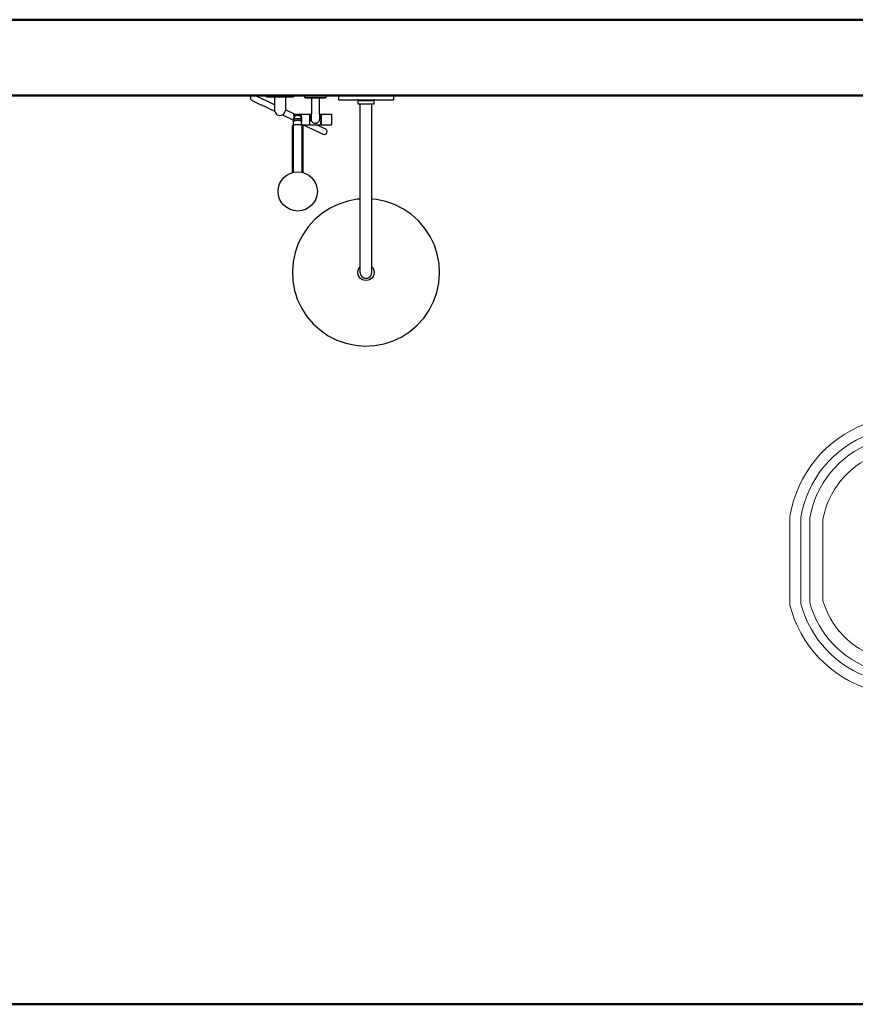
# Model space of a CAD drawing. Units: inches. Extents: x 64 to 1167, y 117 to 939.
# Tile 6 of 56: x 166 to 210, y 585 to 637. Entities that reach past the tile are written whole.
import ezdxf

# ---------------------------------------------------------------- set-up
doc = ezdxf.new("R2010")
doc.units = ezdxf.units.IN
doc.header["$MEASUREMENT"] = 0
doc.layers.add('A-FLOR-FIXT', color=8, linetype='Continuous', lineweight=18)
doc.layers.add('A-WALL', color=7, linetype='Continuous', lineweight=50)
doc.layers.add('Edges', color=7, linetype='Continuous')

# ---------------------------------------------------------------- blocks, each defined once
blk = doc.blocks.new('A$C2B992F40')
for p, q in [((39.23129452295689, 615.2381772181615), (39.23129452295689, 696.1525377148282)), ((39.23129452295689, 696.1525377148282), (475.6793350467342, 696.1525377148282)), ((66.84834779340599, 669.7333433559179), (39.23129452295689, 696.1525377148282)), ((444.2292548016194, 669.7333433559179), (475.6793350467342, 696.1525377148282)), ((475.6793350467342, 696.1525377148282), (475.6793350467342, 509.804294059264)), ((66.84834779340599, 534.621940808509), (66.84834779340599, 669.7333433559179)), ((66.84834779340599, 669.7333433559179), (444.2292548016194, 669.7333433559179)), ((444.2292548016194, 669.7333433559179), (444.2292548016194, 534.621940808509)), ((1.44959776662e-05, 561.2952507389491), (1.44959776662e-05, 615.2381772181615)), ((1.44959776662e-05, 615.2381772181615), (51.49109464316279, 615.2381772181615)), ((51.49109464316279, 615.2381772181615), (51.49109464316279, 556.391369584213)), ((51.49109464316279, 556.391369584213), (39.23129452295689, 553.9393997847291)), ((39.23129452295689, 522.0640261682347), (39.23129452295689, 553.9393997847291)), ((444.2292548016194, 534.621940808509), (66.84834779340599, 534.621940808509)), ((40.05894495480606, 461.2424459844842), (39.23129452295689, 522.0640261682347)), ((475.6793350467342, 509.804294059264), (475.6793350467342, 451.9244464370785)), ((84.15013235549122, 464.3949121413388), (431.5493350467368, 464.3949121413388)), ((129.7295725633375, 113.4341665071333), (84.15013235549122, 464.3949121413388)), ((431.5493350467368, 464.3949121413388), (431.5493350467368, 454.00713756623)), ((449.2013350467313, 464.3949121413388), (449.2013350467313, 453.1740611144559)), ((460.9693350467351, 464.3949121413388), (460.9693350467351, 452.6186768132683)), ((86.64921221682016, 102.498352967923), (40.05894495480606, 461.2424459844842)), ((101.0214604892535, 106.0502375904107), (54.97514125393355, 460.6059420669843)), ((112.5111080790666, 108.954508036426), (66.64513769455516, 462.1215300967232)), ((431.5493350467368, 454.00713756623), (399.5914999541783, 116.1850619918623)), ((449.2013350467313, 453.1740611144559), (416.971452608137, 112.4762087915951)), ((460.9693350467351, 452.6186768132683), (428.565302922565, 110.0799110474254)), ((475.6793350467342, 451.9244464370785), (443.0645039794763, 107.1573527416403)), ((324.1854972264919, 44.13000728074258), (215.003512285366, 44.13000728074258)), ((326.6635935081504, 26.47800728074071), (213.4391771910814, 26.47800728074071)), ((328.2227788998353, 14.71000728074432), (212.454121287592, 14.71000728077342)), ((330.0831719967318, 7.2807524703e-06), (211.2780859033082, 7.2807524703e-06))]:
    blk.add_line(p, q)
for centre, radius, start, end in [((22.20240071017542, 571.4133313514467), 24.39921123490088, 204.4997228087197, 314.2610062863615), ((280.2612989637637, 1327.830131300739), 841.0436844903729, 253.3464205734561, 283.4355732391427), ((60.19932523783428, 466.0669930520307), 7.557458313409357, 328.5293214584837, 226.2699072251538), ((454.4255190306357, 466.066993052038), 7.55745831341713, 328.5293214584293, 226.2699072251538), ((235.9324939092958, 156.9955617533414), 144.2096147714489, 200.687621012972, 260.6301224882377), ((235.9324939114658, 156.9955617559462), 132.4416147714598, 201.268184894862, 260.2217325128458), ((235.9324939129765, 156.9955617578016), 114.7896147714715, 202.302033268819, 259.4948038480974), ((291.5369934622749, 153.7807635527424), 114.4080991410291, 286.5808957318149, 340.815540399485), ((291.5369934625532, 153.7807635524514), 132.0600991410263, 285.425757471148, 341.7737032050673), ((291.5369934642304, 153.7807635506833), 143.8280991410254, 284.7775485235246, 342.3115594880128), ((291.5369934621704, 153.7807635528807), 158.5380991410149, 284.0716514048067, 342.8974225244143), ((235.9324939112266, 156.9955617556625), 158.9196147714513, 200.0550662279381, 261.0752231753924)]:
    blk.add_arc(centre, radius, start, end)
blk = doc.blocks.new('Handheld Shower set pl')
at = {"layer": 'Edges'}
for p, q in [((254.88782610443, 328.7344486722934), (274.2130075602099, 319.5581778553694)), ((262.0378967387861, 340.8240422599073), (280.2128437873457, 332.1939428953848)), ((287.6357447226078, 328.6692903903087), (280.2128437873457, 332.1939428953848)), ((280.2128437873457, 332.1939428953848), (282.6934018041104, 331.0160873502237)), ((308.3053185319595, 318.8546551498083), (287.6357447226078, 328.6692903903087)), ((352.8381736068126, 340.8480149876004), (289.3381736068126, 340.848014987464)), ((289.3381736068126, 340.848014987464), (289.3381736068194, 337.6730149874711)), ((289.3381736068194, 337.6730149874711), (308.3881736068245, 337.6730149875027)), ((308.3881736068245, 337.6730149875027), (308.3881736068652, 318.8156109906679)), ((308.3881736068245, 337.6730149875027), (333.7881736068244, 337.6730149875565)), ((333.7881736068244, 337.6730149875565), (333.7881736068912, 306.7548869674145)), ((333.7881736068244, 337.6730149875565), (352.8381736068194, 337.6730149876075)), ((352.8381736068126, 340.8480149876004), (352.8381736068194, 337.6730149876075)), ((379.7084284701686, 340.4511399876282), (379.7084284701771, 336.4823899876282)), ((380.056935936017, 340.6883716268995), (430.15992100432, 340.6883716270087)), ((380.056935936017, 336.2451583485752), (430.15992100432, 336.245158348466)), ((381.5890066633125, 335.2861388397479), (428.8429137266978, 335.2861388397479)), ((395.583428470181, 335.2861388397479), (395.5834284702646, 296.3729544387613)), ((414.6334284702645, 296.3729544388023), (414.6334284701809, 335.2861388397479)), ((430.5084284701685, 340.4511399877374), (430.508428470177, 336.4823899877373)), ((460.0631736067644, 340.848014987583), (460.0631736067644, 330.7230149875665)), ((591.6881736068635, 340.8480149875829), (460.0631736067644, 340.848014987583)), ((460.0631736067644, 330.7230149875665), (505.5244174469552, 330.7230149875665)), ((505.7322518774402, 330.6816984589821), (505.5244174469552, 330.7230149875665)), ((505.9329121943118, 330.6135834691153), (505.7322518774402, 330.6816984589821)), ((505.7322518774402, 330.6816984589821), (545.5961902985603, 330.6816984162817)), ((506.1229650436863, 330.5198597845081), (505.9329121943118, 330.6135834691153)), ((506.2991585684015, 330.4021310434972), (506.1229650436863, 330.5198597845081)), ((506.458478048199, 330.2624116176158), (506.2991585684015, 330.4021310434972)), ((506.598197482426, 330.1030921451366), (506.458478048199, 330.2624116176158)), ((506.7159262326659, 329.9268986265877), (506.598197482426, 330.1030921451366)), ((506.8096499272279, 329.7368457821227), (506.7159262326659, 329.9268986265877)), ((506.8777649276057, 329.5361854688187), (506.8096499272279, 329.7368457821227)), ((506.9191057671805, 329.3283510404998), (506.8777649276057, 329.5361854688187)), ((506.9329650926778, 329.1168986020924), (506.9191057671805, 329.3283510404998)), ((544.3954772426832, 329.1168984607566), (506.9329650926778, 329.1168986020924)), ((506.9462863494702, 320.4087238914977), (506.9462802744978, 328.9137481916184)), ((506.9462802744978, 328.9137481916184), (544.4087924245033, 328.9137480502832)), ((544.4093365494242, 329.3283508980291), (544.3954772426832, 329.1168984607566)), ((544.4087924245033, 328.9137480502832), (544.4087863495309, 320.4087238914977)), ((544.450677369951, 329.5361853277313), (544.4093365494242, 329.3283508980291)), ((544.5187923513319, 329.736845644992), (544.450677369951, 329.5361853277313)), ((544.612516027298, 329.926898495996), (544.5187923513319, 329.736845644992)), ((544.7302447596979, 330.1030920236273), (544.612516027298, 329.926898495996)), ((544.8699641771904, 330.2624115076441), (544.7302447596979, 330.1030920236273)), ((545.0292836416982, 330.4021309473805), (544.8699641771904, 330.2624115076441)), ((545.2054771528917, 330.5198597043816), (545.0292836416982, 330.4021309473805)), ((545.3955299908102, 330.6135834068843), (545.2054771528917, 330.5198597043816)), ((545.5961902985603, 330.6816984162817), (545.3955299908102, 330.6135834068843)), ((545.8040247224903, 330.7230149875664), (545.5961902985603, 330.6816984162817)), ((545.8040247224903, 330.7230149875664), (591.6881736068635, 330.7230149875664)), ((591.6881736068635, 330.7230149875664), (591.6881736068635, 340.8480149875829)), ((274.2130075602099, 319.5581778553694), (276.6781894745287, 318.3955521668955)), ((279.5594820654953, 317.0196883363817), (276.6781894745287, 318.3955521668955)), ((279.5594820654953, 317.0196883363817), (281.6359083981089, 316.033525396527)), ((294.8483957772038, 309.7597751275736), (281.6359083981089, 316.033525396527)), ((294.8483957772038, 309.7597751275736), (308.7522275987269, 303.1577503818214)), ((308.3053185319595, 318.8546551498083), (308.3881736068652, 318.8156109906679)), ((308.3881736068652, 318.8156109906679), (308.388173606893, 305.9230149874992)), ((308.388173606893, 305.9230149874992), (308.7522275987269, 303.1577503818214)), ((333.3554316007712, 302.6360131147537), (333.788173606893, 305.9230149875566)), ((333.7881736068912, 306.7548869674145), (333.788173606893, 305.9230149875566)), ((355.6525909409219, 296.3729544386691), (333.7881736068912, 306.7548869674145)), ((511.4015080443246, 320.4087238914977), (506.9462863494702, 320.4087238914977)), ((511.4015080443246, 94.2362761450968), (511.4015080443246, 320.4087238914977)), ((539.4015080443241, 320.4087238914977), (511.4015080443246, 320.4087238914977)), ((539.401508044324, 94.16884688835617), (539.4015080443241, 320.4087238914977)), ((544.4087863495309, 320.4087238914977), (539.4015080443241, 320.4087238914977)), ((308.7522275987269, 303.1577503818214), (308.8209156130289, 302.6360131146978)), ((308.8209156130289, 302.6360131146978), (310.0896509788445, 299.5730149875021)), ((310.0896509788445, 299.5730149875021), (312.107917485843, 296.9427588664379)), ((312.107917485843, 296.9427588664379), (314.7381736069166, 294.92449235945)), ((314.7381736069166, 294.92449235945), (317.8011717341174, 293.6557569936479)), ((317.8011717341174, 293.6557569936479), (321.0881736069203, 293.2230149875264)), ((321.0881736069203, 293.2230149875264), (324.3751754797212, 293.655756993662)), ((324.3751754797212, 293.655756993662), (326.7193112154868, 294.6267298074699)), ((326.7193112154868, 294.6267298074699), (327.4381736069166, 294.9244923594772)), ((326.7193112154868, 294.6267298074699), (352.864355566542, 282.2122164068355)), ((327.4381736069166, 294.9244923594772), (330.0684297279815, 296.9427588664765)), ((330.0684297279815, 296.9427588664765), (332.0866962349688, 299.5730149875494)), ((332.0866962349688, 299.5730149875494), (333.3554316007712, 302.6360131147537)), ((352.9209557304838, 285.6318500002028), (352.7585192937348, 284.3460332032719)), ((352.7585192937348, 284.3460332032719), (352.7585192937376, 283.0499967719733)), ((352.7585192937376, 283.0499967719733), (352.864355566542, 282.2122164068355)), ((352.864355566542, 282.2122164068355), (352.9209557304922, 281.7641799750433)), ((353.2432668843423, 286.8871690637685), (352.9209557304838, 285.6318500002028)), ((352.9209557304922, 281.7641799750433), (353.2432668843561, 280.5088609114788)), ((353.7203697158746, 288.0921932624454), (353.2432668843423, 286.8871690637685)), ((353.5146784702647, 296.3729544386645), (355.6525909409219, 296.3729544386691)), ((353.5146784702647, 296.3729544386645), (353.5146784702714, 293.2230149876263)), ((353.5146784702714, 293.2230149876263), (359.109298929503, 293.2230149876383)), ((353.7021878188209, 285.4828220090641), (353.5522692937349, 284.2960946861515)), ((353.5522692937377, 282.9904534152568), (353.5522692937349, 284.2960946861515)), ((353.5522692937377, 282.9904534152568), (353.6272285562831, 282.506571627662)), ((353.5522692937377, 282.9904534152568), (353.5522692937401, 281.8648279686577)), ((353.5522692937401, 281.8648279686577), (353.627228556284, 282.0585375299411)), ((353.6272285562857, 281.2999859419838), (353.5522692937401, 281.8648279686577)), ((353.5522692937428, 279.7284099140281), (353.5522692937401, 281.8648279686577)), ((353.6272285562831, 282.506571627662), (353.850924191566, 282.9856041258255)), ((353.627228556284, 282.0585375299411), (353.6272285562831, 282.506571627662)), ((353.627228556284, 282.0585375299411), (353.6272285562857, 281.2999859419838)), ((353.9996605642978, 286.6414018590571), (353.7021878188209, 285.4828220090641)), ((354.3447400284199, 289.227918644774), (353.7203697158746, 288.0921932624454)), ((353.850924191566, 282.9856041258255), (354.2198283857908, 283.5238629468017)), ((354.439996207268, 287.753562739794), (353.9996605642978, 286.6414018590571)), ((354.2198283857908, 283.5238629468017), (354.728123299442, 284.0359577951134)), ((355.1065311291687, 290.2764341430252), (354.3447400284199, 289.227918644774)), ((355.0162503915978, 288.8017652098128), (354.439996207268, 287.753562739794)), ((354.728123299442, 284.0359577951134), (355.3677928180907, 284.5138126290921)), ((355.719335244563, 289.7694784899957), (355.0162503915978, 288.8017652098128)), ((355.0162503916127, 280.528170801557), (355.7193352445791, 280.9371441058922)), ((355.9937291173903, 291.221204041439), (355.1065311291687, 290.2764341430252)), ((355.3677928180907, 284.5138126290921), (356.1287489713077, 284.9498913925493)), ((355.6525909409219, 296.3729544386691), (391.2178034702647, 296.3729544387455)), ((356.5381626980298, 290.6414411638301), (355.719335244563, 289.7694784899957)), ((355.7193352445791, 280.9371441058922), (356.538162698047, 281.3056514554121)), ((356.9923423508239, 292.0473287543392), (355.9937291173903, 291.221204041439)), ((356.1287489713077, 284.9498913925493), (356.9989910259837, 285.3373168628847)), ((357.4598193539131, 291.4039018590646), (356.5381626980298, 290.6414411638301)), ((356.538162698047, 281.3056514554121), (357.4598193539312, 281.6278812690788)), ((358.0866221022359, 292.7417798015003), (356.9923423508239, 292.0473287543392)), ((356.9989910259837, 285.3373168628847), (357.964794745059, 285.669979108994)), ((358.4697701361788, 292.0448361150631), (357.4598193539131, 291.4039018590646)), ((357.4598193539312, 281.6278812690788), (358.4697701361977, 281.8987517902403)), ((357.964794745059, 285.669979108994), (359.0109288269405, 285.9426318485333)), ((359.109298929503, 293.2230149876383), (358.0866221022359, 292.7417798015003)), ((359.5520875176749, 292.5541360157333), (358.4697701361788, 292.0448361150631)), ((358.4697701361977, 281.8987517902403), (359.5520875176944, 282.1139912289676)), ((359.0109288269405, 285.9426318485333), (360.1208951122268, 286.1509751849255)), ((359.2593109262551, 293.2936052750667), (359.109298929503, 293.2230149876383)), ((360.4919148195967, 293.6941025576697), (359.2593109262551, 293.2936052750667)), ((360.6897027067504, 292.9237695974003), (359.5520875176749, 292.5541360157333)), ((359.5520875176944, 282.1139912289676), (360.6897027067704, 282.2702051307341)), ((360.1208951122268, 286.1509751849255), (361.2771887695373, 286.2917234192971)), ((361.7649948825407, 293.9369555679202), (360.4919148195967, 293.6941025576697)), ((361.8646748322952, 293.1479075176731), (360.6897027067504, 292.9237695974003)), ((360.6897027067704, 282.2702051307341), (361.8646748323155, 282.3649299089916)), ((361.2771887695373, 286.2917234192971), (362.4615743571598, 286.3626568679134)), ((363.0584738819933, 294.0183343687731), (361.7649948825407, 293.9369555679202)), ((363.058473881995, 293.2230149876552), (361.8646748322952, 293.1479075176731)), ((361.8646748323155, 282.3649299089916), (363.0584738820154, 282.3966716974006)), ((362.4615743571598, 286.3626568679134), (363.6553734068598, 286.3626568679159)), ((363.0584738819936, 292.9207316193203), (363.0584738819849, 297.0751597092863)), ((364.3519528814463, 293.9369555679257), (363.0584738819933, 294.0183343687731)), ((364.2522729316952, 293.1479075176781), (363.058473881995, 293.2230149876552)), ((364.2522729317154, 282.3649299089966), (363.0584738820154, 282.3966716974006)), ((363.6553734068598, 286.3626568679159), (364.8397589944825, 286.2917234193048)), ((365.427245057241, 292.9237695974105), (364.2522729316952, 293.1479075176781)), ((364.2522729317154, 282.3649299089966), (365.427245057261, 282.2702051307443)), ((365.6250329443913, 293.6941025576807), (364.3519528814463, 293.9369555679257)), ((364.8397589944825, 286.2917234193048), (365.9960526517937, 286.150975184938)), ((366.5648602463181, 292.5541360157483), (365.427245057241, 292.9237695974105)), ((365.427245057261, 282.2702051307443), (366.5648602463376, 282.1139912289826)), ((366.8576368377346, 293.2936052750831), (365.6250329443913, 293.6941025576807)), ((365.9960526517937, 286.150975184938), (367.1060189370809, 285.9426318485507)), ((367.6471776278164, 292.0448361150828), (366.5648602463181, 292.5541360157483)), ((366.5648602463376, 282.1139912289826), (367.6471776278353, 281.8987517902601)), ((367.0076488344871, 293.2230149876553), (366.8576368377346, 293.2936052750831)), ((368.0303256617563, 292.7417798015217), (367.0076488344871, 293.2230149876553)), ((367.0076488344871, 293.2230149876553), (372.5646784702715, 293.2230149876673)), ((367.1060189370809, 285.9426318485507), (368.1521530189636, 285.6699791090158)), ((368.6571284100848, 291.4039018590886), (367.6471776278164, 292.0448361150828)), ((367.6471776278353, 281.8987517902601), (368.6571284101029, 281.6278812691029)), ((369.1246054131712, 292.0473287543653), (368.0303256617563, 292.7417798015217)), ((368.1521530189636, 285.6699791090158), (369.1179567380403, 285.3373168629107)), ((369.5787850659714, 290.6414411638581), (368.6571284100848, 291.4039018590886)), ((368.6571284101029, 281.6278812691029), (369.5787850659885, 281.30565145544)), ((369.1179567380403, 285.3373168629107), (369.9881987927179, 284.9498913925791)), ((370.1232186466084, 291.2212040414694), (369.1246054131712, 292.0473287543653)), ((370.3976125194419, 289.7694784900273), (369.5787850659714, 290.6414411638581)), ((369.5787850659885, 281.30565145544), (370.3976125194579, 280.9371441059239)), ((369.9881987927179, 284.9498913925791), (370.7491549459368, 284.5138126291251)), ((371.010416634834, 290.2764341430594), (370.1232186466084, 291.2212040414694)), ((371.1006973724112, 288.8017652098474), (370.3976125194419, 289.7694784900273)), ((370.3976125194579, 280.9371441059239), (371.1006973724261, 280.5281708015916)), ((370.7491549459368, 284.5138126291251), (371.3888244645876, 284.0359577951492)), ((371.7722077355873, 289.2279186448114), (371.010416634834, 290.2764341430594)), ((371.6769515567456, 287.753562739831), (371.1006973724112, 288.8017652098474)), ((371.3888244645876, 284.0359577951492), (371.897119378241, 283.5238629468397)), ((372.1172871997205, 286.641401859096), (371.6769515567456, 287.753562739831)), ((372.1509484088954, 288.5389919175999), (371.7722077355873, 289.2279186448114)), ((371.897119378241, 283.5238629468397), (372.266023572468, 282.9856041258651)), ((372.4147599452024, 285.4828220091043), (372.1172871997205, 286.641401859096)), ((372.5646784702819, 288.3425390948654), (372.1509484088954, 288.5389919175999)), ((372.3965780481375, 288.0921932624856), (372.1509484088954, 288.5389919175999)), ((372.266023572468, 282.9856041258651), (372.4897192077531, 282.506571627698)), ((372.2660235724716, 281.3339180412498), (372.4147599452101, 281.9132079662462)), ((372.2660235724729, 280.7440518115306), (372.4897192077557, 281.2999859420244)), ((372.5646784702834, 287.6676200612735), (372.3965780481375, 288.0921932624856)), ((372.5646784702935, 284.2960946861923), (372.4147599452024, 285.4828220091043)), ((372.4147599452101, 281.9132079662462), (372.4897192077535, 282.2988956940436)), ((372.4897192077531, 282.506571627698), (372.5646784702963, 282.9904534152976)), ((372.4897192077531, 282.506571627698), (372.4897192077535, 282.2988956940436)), ((372.489719207754, 282.0585375299815), (372.4897192077535, 282.2988956940436)), ((372.489719207754, 282.0585375299815), (372.5646784702988, 281.8648279686986)), ((372.489719207754, 282.0585375299815), (372.4897192077557, 281.2999859420244)), ((372.5646784702988, 281.8648279686986), (372.4897192077557, 281.2999859420244)), ((372.5646784702819, 288.3425390948654), (372.5646784702715, 293.2230149876673)), ((372.5646784702819, 288.3425390948654), (372.5646784702834, 287.6676200612735)), ((372.873680879675, 286.8871690638138), (372.5646784702834, 287.6676200612735)), ((372.5646784702963, 282.9904534152976), (372.5646784702935, 284.2960946861923)), ((372.5646784702963, 282.9904534152976), (372.5646784702988, 281.8648279686986)), ((372.5646784702988, 281.8648279686986), (372.5646784703005, 279.7284099140569)), ((373.1959920335389, 285.6318500002494), (372.873680879675, 286.8871690638138)), ((372.8736808796887, 280.5088609115241), (373.1959920335472, 281.7641799750898)), ((373.3584284702934, 284.3460332033193), (373.1959920335389, 285.6318500002494)), ((373.1959920335472, 281.7641799750898), (373.3584284702962, 283.0499967720207)), ((373.3584284702962, 283.0499967720207), (373.3584284702934, 284.3460332033193)), ((391.591996008745, 295.9788423783764), (391.591996008745, 271.4171875970299)), ((391.9855966033532, 295.5816204628969), (391.591996008745, 295.5816204628969)), ((391.9855966033532, 295.5816204628969), (391.9855966033881, 279.3147186037287)), ((392.0115534702664, 295.5807707230573), (392.0115534703018, 279.1085107151291)), ((393.2021784702647, 296.3729544387563), (395.5834284702646, 296.3729544387613)), ((395.583428470292, 283.6980149877519), (395.5834284702646, 296.3729544387613)), ((395.6585359402741, 282.5042159380522), (395.583428470292, 283.6980149877519)), ((395.8826738605468, 281.3292438125076), (395.6585359402741, 282.5042159380522)), ((396.2523074422139, 280.1916286234322), (395.8826738605468, 281.3292438125076)), ((414.3341830800472, 281.3292438125472), (413.9645494983851, 280.1916286234702)), ((414.5583210003149, 282.5042159380928), (414.3341830800472, 281.3292438125472)), ((414.6334284702919, 283.6980149877928), (414.5583210003149, 282.5042159380928)), ((414.6334284702645, 296.3729544388023), (417.0146784702646, 296.3729544388074)), ((414.6334284702645, 296.3729544388023), (414.6334284702919, 283.6980149877928)), ((418.2053034703718, 295.5807707231084), (418.2053034703365, 279.1085107151803)), ((418.231260337285, 295.581620462948), (418.2312603372501, 279.3147186037799)), ((418.231260337285, 295.581620462948), (418.6248609318933, 295.581620462948)), ((418.6248609318933, 295.9788423784275), (418.6248609318933, 271.4171875970811)), ((418.9990534704, 296.3729544388111), (443.2084284702646, 296.3729544388631)), ((443.9181109627157, 271.9899216200651), (443.9181109627157, 295.4061083558726)), ((350.3584738820491, 266.8611238589264), (350.4586171753537, 267.6010884018294)), ((350.3584738820491, 266.8611238589264), (350.3584738822842, 157.5124257988244)), ((350.4586171753537, 267.6010884018294), (350.7574677357123, 268.3293832618582)), ((350.7574677357123, 268.3293832618582), (351.2503125112637, 269.0345227940073)), ((351.2503125112637, 269.0345227940073), (351.929379045486, 269.7053865266251)), ((351.929379045486, 269.7053865266251), (352.7839580534799, 270.3313945378936)), ((352.7839580534799, 270.3313945378936), (353.1489329823415, 270.5364898246886)), ((353.254177407083, 270.6620795897073), (353.1489329823413, 270.6182002058067)), ((353.1489329823415, 270.5364898246886), (353.1489329823413, 270.6182002058067)), ((353.1489329823573, 263.1857578931758), (353.1489329823415, 270.5364898246886)), ((353.148932982582, 158.2215903391118), (353.1489329823573, 263.1857578931758)), ((353.2432668843561, 280.5088609114788), (353.5522692937428, 279.7284099140281)), ((353.3684326937872, 270.7057710753496), (353.254177407083, 270.6620795897073)), ((353.4912095837754, 270.7490875690844), (353.3684326937872, 270.7057710753496)), ((353.552269293764, 270.7631420408396), (353.4912095837754, 270.7490875690844)), ((353.5146784703124, 274.1730149876263), (353.5522692937453, 278.1184733517295)), ((353.5146784703187, 271.2229669033708), (353.5146784703124, 274.1730149876263)), ((353.5146784703124, 274.1730149876263), (353.6272285563009, 274.1730149876265)), ((353.5146784703187, 271.2229669033708), (353.5146784703191, 271.0230755365862)), ((353.5522692937634, 271.0230755365864), (353.5146784703187, 271.2229669033708)), ((353.5146784703191, 271.0230755365862), (353.5522692937634, 271.0230755365864)), ((353.5522692937428, 279.7284099140281), (353.6272285562894, 279.5390844283831)), ((353.5522692937442, 278.6239921568687), (353.5522692937428, 279.7284099140281)), ((353.7021878188317, 279.1255247952384), (353.5522692937442, 278.6239921568687)), ((353.5522692937442, 278.6239921568687), (353.5522692937453, 278.1184733517295)), ((353.5522692937453, 278.1184733517295), (353.627228556293, 277.8677070325352)), ((353.5774142949124, 270.7772721106449), (353.5522692937634, 271.0230755365864)), ((353.5774142949124, 270.7772721106449), (353.552269293764, 270.7631420408396)), ((353.8005723137885, 270.902674307516), (353.5774142949124, 270.7772721106449)), ((353.5774142949124, 270.7772721106449), (353.6219823275558, 270.7918435830354)), ((353.6219823275558, 270.7918435830354), (353.8005723137885, 270.902674307516)), ((353.7021878188317, 279.1255247952384), (353.99966056431, 279.6151617975308)), ((353.8005723137885, 270.902674307516), (353.8005723137886, 270.845294837962)), ((353.8005723137886, 270.845294837962), (353.9052435791159, 270.874945004394)), ((353.9052435791159, 270.874945004394), (354.0565191187296, 270.9149345587573)), ((353.99966056431, 279.6151617975308), (354.4399962072815, 280.0851812957245)), ((354.0565191187296, 270.9149345587573), (354.2133697699187, 270.9536534510659)), ((354.2133697699187, 270.9536534510659), (354.3751238741147, 270.9909358810784)), ((354.3751238741147, 270.9909358810784), (354.5410887754106, 271.026622199706)), ((354.4399962072815, 280.0851812957245), (355.0162503916127, 280.528170801557)), ((354.5410887754106, 271.026622199706), (354.7105537866196, 271.0605595926537)), ((354.7105537866196, 271.0605595926537), (354.8827932325469, 271.0926027347946)), ((354.8827932325469, 271.0926027347946), (355.0570695574425, 271.1226144124749)), ((355.0570695574425, 271.1226144124749), (355.2326364833276, 271.1504661110831)), ((355.2326364833276, 271.1504661110831), (355.4087422056722, 271.1760385653702)), ((355.4087422056722, 271.1760385653702), (355.584632612737, 271.1992222701605)), ((355.584632612737, 271.1992222701605), (355.7595545147956, 271.2199179492712)), ((355.7595545147956, 271.2199179492712), (355.932758869409, 271.2380369806272)), ((355.932758869409, 271.2380369806272), (356.10350398894, 271.2535017757541)), ((356.10350398894, 271.2535017757541), (356.2710587165733, 271.2662461120254)), ((356.2710587165733, 271.2662461120254), (356.4347055572418, 271.2762154162364)), ((356.5937437500504, 271.2833669982962), (356.4347055572418, 271.2762154162364)), ((356.7474922690412, 271.2876702340321), (356.5937437500504, 271.2833669982962)), ((356.8952927394522, 271.2891066963283), (356.7474922690412, 271.2876702340321)), ((369.2216550246274, 271.2891066963548), (356.8952927394522, 271.2891066963283)), ((369.3694554950385, 271.2876702340592), (369.2216550246274, 271.2891066963548)), ((369.5232040140293, 271.2833669983239), (369.3694554950385, 271.2876702340592)), ((369.5232040140293, 271.2833669983239), (369.6822422068377, 271.2762154162649)), ((369.6822422068377, 271.2762154162649), (369.8458890475063, 271.2662461120546)), ((369.8458890475063, 271.2662461120546), (370.0134437751397, 271.253501775784)), ((370.0134437751397, 271.253501775784), (370.1841888946706, 271.2380369806577)), ((370.1841888946706, 271.2380369806577), (370.357393249284, 271.2199179493026)), ((370.357393249284, 271.2199179493026), (370.5323151513427, 271.1992222701927)), ((370.5323151513427, 271.1992222701927), (370.7082055584075, 271.176038565403)), ((370.7082055584075, 271.176038565403), (370.8843112807522, 271.1504661111168)), ((370.8843112807522, 271.1504661111168), (371.0598782066374, 271.1226144125094)), ((371.0598782066374, 271.1226144125094), (371.234154531533, 271.0926027348298)), ((371.1006973724261, 280.5281708015916), (371.6769515567592, 280.0851812957616)), ((371.234154531533, 271.0926027348298), (371.4063939774604, 271.0605595926895)), ((371.4063939774604, 271.0605595926895), (371.5758589886694, 271.0266221997426)), ((371.5758589886694, 271.0266221997426), (371.7418238899655, 270.9909358811156)), ((371.6769515567592, 280.0851812957616), (372.1172871997327, 279.6151617975697)), ((371.7418238899655, 270.9909358811156), (371.9035779941616, 270.9536534511039)), ((371.9035779941616, 270.9536534511039), (372.0604286453508, 270.914934558796)), ((372.0604286453508, 270.914934558796), (372.2117041849646, 270.8749450044335)), ((372.1172871997327, 279.6151617975697), (372.3537539651887, 279.2259399951074)), ((372.2117041849646, 270.8749450044335), (372.3163754502925, 270.8452948380017)), ((372.2660235724801, 277.3721222122591), (372.4147599452165, 277.6169407134005)), ((372.266023572487, 274.1730149876667), (372.5646784703124, 274.1730149876672)), ((372.2660235724938, 271.0230755366265), (372.564678470322, 271.0230755366272)), ((372.3163754502924, 270.9026743075557), (372.3163754502925, 270.8452948380017)), ((372.3163754502924, 270.9026743075557), (372.5395334691701, 270.7772721106851)), ((372.3163754502925, 270.8452948380017), (372.3567568279179, 270.8338560294271)), ((372.3537539651887, 279.2259399951074), (372.3965780481564, 279.3038367128471)), ((372.4147599452132, 279.1255247952787), (372.3537539651887, 279.2259399951074)), ((372.3567568279179, 270.8338560294271), (372.4949654365249, 270.7918435830761)), ((372.3965780481564, 279.3038367128471), (372.5646784703005, 279.7284099140569)), ((372.5646784703028, 278.6239921569096), (372.4147599452132, 279.1255247952787)), ((372.4147599452165, 277.6169407134005), (372.5646784703039, 278.1184733517703)), ((372.4949654365249, 270.7918435830761), (372.5395334691701, 270.7772721106851)), ((372.5395334691701, 270.7772721106851), (372.5646784703226, 270.7631420408777)), ((372.5646784703005, 279.7284099140569), (372.8736808796887, 280.5088609115241)), ((372.5646784703005, 279.7284099140569), (372.5646784703028, 278.6239921569096)), ((372.5646784703039, 278.1184733517703), (372.5646784703028, 278.6239921569096)), ((372.5646784703124, 274.1730149876672), (372.5646784703039, 278.1184733517703)), ((372.5646784703124, 274.1730149876672), (372.564678470322, 271.0230755366272)), ((372.564678470322, 271.0230755366272), (376.4286024379837, 271.0230755366357)), ((372.564678470322, 271.0230755366272), (372.5646784703226, 270.7631420408777)), ((372.5646784703226, 270.7631420408777), (372.6257381803053, 270.7490875691255)), ((372.6257381803053, 270.7490875691255), (372.7485150702938, 270.7057710753913)), ((372.7485150702938, 270.7057710753913), (372.8627703569981, 270.6620795897495)), ((372.7485150702938, 270.7057710753913), (372.7485150702938, 270.6598362595415)), ((372.7485150702938, 270.6598362595415), (372.8627703569982, 270.5956312445084)), ((372.8627703569981, 270.6620795897495), (372.96801478174, 270.6182002058493)), ((372.8627703569981, 270.6620795897495), (372.8627703569982, 270.5956312445084)), ((372.8627703569982, 270.5956312445084), (372.9680147817402, 270.5364898247317)), ((372.96801478174, 270.6182002058493), (372.9680147817402, 270.5364898247317)), ((372.9680147817402, 270.5364898247317), (372.9680147819814, 158.2964037718719)), ((372.9680147817402, 270.5364898247317), (373.3329897106036, 270.3313945379377)), ((373.3329897106036, 270.3313945379377), (374.1875687186001, 269.705386526673)), ((374.1875687186001, 269.705386526673), (374.8666352528253, 269.034522794058)), ((374.8666352528253, 269.034522794058), (375.3594800283796, 268.329383261911)), ((375.3594800283796, 268.329383261911), (375.6583305887414, 267.6010884018836)), ((375.6583305887414, 267.6010884018836), (375.7584738820491, 266.8611238589808)), ((375.7584738820491, 266.8611238589808), (375.7584738822838, 157.6097980131866)), ((376.4286024379837, 271.0230755366357), (391.2178034703192, 271.0230755366672)), ((376.4286024379837, 271.0230755366357), (423.3542027044977, 248.7411623097145)), ((391.9855966034043, 271.8144095125191), (391.5919960087449, 271.8144095125191)), ((391.959750887764, 279.3137796601437), (391.9855966033886, 279.120835922249)), ((391.9855966033886, 279.120835922249), (391.9597508877643, 279.1331083509399)), ((391.9855966033886, 279.120835922249), (391.9597508877669, 277.9604963631635)), ((391.9855966033881, 279.3147186037287), (392.0115534703018, 279.1085107151291)), ((392.0115534703018, 279.1085107151291), (391.9855966033886, 279.120835922249)), ((392.0115534703018, 279.1085107151291), (391.9855966033911, 277.9617251307601)), ((391.9855966034043, 271.8144095125191), (391.9855966033911, 277.9617251307601)), ((391.9855966034043, 271.8144095125191), (392.0115534703175, 271.8152592523589)), ((392.0115534703175, 271.8152592523589), (392.0115534703018, 279.1085107151291)), ((392.0115534703175, 271.8152592523589), (392.4084284703174, 271.8152592523598)), ((392.0115534703175, 271.815259252359), (392.4084284703174, 271.81525925236)), ((392.4101279499969, 271.7649118028498), (392.4084284703174, 271.8168255366763)), ((392.4152191116022, 271.7132203716017), (392.4101279499969, 271.7649118028498)), ((392.4236801539977, 271.661972593576), (392.4152191116022, 271.7132203716017)), ((392.4354748457009, 271.6113879196263), (392.4236801539977, 271.661972593576)), ((392.4505526800313, 271.561682961092), (392.4354748457009, 271.6113879196263)), ((392.4688490913873, 271.5130705622367), (392.4505526800313, 271.561682961092)), ((392.4902857317267, 271.4657588888151), (392.4688490913873, 271.5130705622367)), ((392.5147708060644, 271.4199505366766), (392.4902857317267, 271.4657588888151)), ((392.5421994655533, 271.3758416642173), (392.5147708060644, 271.4199505366766)), ((392.5724542564623, 271.3336211524009), (392.5421994655533, 271.3758416642173)), ((392.6054056231322, 271.2934697959411), (392.5724542564623, 271.3336211524009)), ((392.6409124627518, 271.25555952911), (392.6054056231322, 271.2934697959411)), ((392.678822729583, 271.2200526894904), (392.6409124627518, 271.25555952911)), ((392.7189740860431, 271.1871013228208), (392.678822729583, 271.2200526894904)), ((392.7611945978595, 271.1568465319119), (392.7189740860431, 271.1871013228208)), ((392.8053034703189, 271.1294178724232), (392.7611945978595, 271.1568465319119)), ((392.8511118224576, 271.1049327980857), (392.8053034703189, 271.1294178724232)), ((392.8984234958792, 271.0834961577465), (392.8511118224576, 271.1049327980857)), ((392.9470358947347, 271.0651997463907), (392.8984234958792, 271.0834961577465)), ((392.996740853269, 271.0501219120606), (392.9470358947347, 271.0651997463907)), ((393.0473255272188, 271.0383272203576), (392.996740853269, 271.0501219120606)), ((393.0473255272188, 271.0383272203576), (393.0985733052445, 271.0298661779623)), ((393.0985733052445, 271.0298661779623), (393.1502647364927, 271.0247750163572)), ((393.1502647364927, 271.0247750163572), (393.2021784703191, 271.023075536678)), ((393.2021784703191, 271.023075536678), (409.0392980331906, 271.0230755367122)), ((396.761607342884, 279.1093112419361), (396.2523074422139, 280.1916286234322)), ((397.4025415988826, 278.0993604596706), (396.761607342884, 279.1093112419361)), ((398.165002294117, 277.1777038037874), (397.4025415988826, 278.0993604596706)), ((399.0369649679515, 276.3588763503208), (398.165002294117, 277.1777038037874)), ((400.0046782481343, 275.6557914973556), (399.0369649679515, 276.3588763503208)), ((401.0528807181531, 275.0795373130257), (400.0046782481343, 275.6557914973556)), ((402.16504159889, 274.6392016700557), (401.0528807181531, 275.0795373130257)), ((403.323621448883, 274.3417289245788), (402.16504159889, 274.6392016700557)), ((404.5103487717956, 274.1918103994929), (403.323621448883, 274.3417289245788)), ((405.706508168829, 274.1918103994954), (404.5103487717956, 274.1918103994929)), ((406.893235491741, 274.3417289245865), (405.706508168829, 274.1918103994954)), ((408.0518153417328, 274.6392016700684), (406.893235491741, 274.3417289245865)), ((409.1639762224677, 275.0795373130432), (408.0518153417328, 274.6392016700684)), ((409.0392980331906, 271.0230755367122), (417.0146784703191, 271.0230755367291)), ((409.0392980331906, 271.0230755367122), (429.3540921681506, 261.3769020713321)), ((410.2121786924841, 275.6557914973775), (409.1639762224677, 275.0795373130432)), ((411.179891972664, 276.3588763503468), (410.2121786924841, 275.6557914973775)), ((412.0518546464949, 277.1777038038173), (411.179891972664, 276.3588763503468)), ((412.8143153417253, 278.0993604597037), (412.0518546464949, 277.1777038038173)), ((413.4552495977196, 279.1093112419719), (412.8143153417253, 278.0993604597037)), ((413.9645494983851, 280.1916286234702), (413.4552495977196, 279.1093112419719)), ((417.0665922041456, 271.0247750164084), (417.0146784703191, 271.0230755367291)), ((417.1182836353938, 271.0298661780135), (417.0665922041456, 271.0247750164084)), ((417.1695314134195, 271.0383272204087), (417.1182836353938, 271.0298661780135)), ((417.1695314134195, 271.0383272204087), (417.2201160873693, 271.0501219121117)), ((417.2201160873693, 271.0501219121117), (417.2698210459036, 271.0651997464418)), ((417.2698210459036, 271.0651997464418), (417.318433444759, 271.0834961577977)), ((417.318433444759, 271.0834961577977), (417.3657451181806, 271.1049327981368)), ((417.3657451181806, 271.1049327981368), (417.5759444778864, 271.2555595291611)), ((417.5759444778864, 271.2555595291611), (417.6114513175061, 271.2934697959922)), ((417.6114513175061, 271.2934697959922), (417.6444026841759, 271.3336211524521)), ((417.6444026841759, 271.3336211524521), (417.674657475085, 271.3758416642685)), ((417.674657475085, 271.3758416642685), (417.7020861345739, 271.4199505367277)), ((417.7020861345739, 271.4199505367277), (417.7265712089116, 271.4657588888663)), ((417.7265712089116, 271.4657588888663), (417.748007849251, 271.5130705622878)), ((417.748007849251, 271.5130705622878), (417.766304260607, 271.5616829611432)), ((417.766304260607, 271.5616829611432), (417.7813820949373, 271.6113879196774)), ((417.7813820949373, 271.6113879196774), (417.7931767866406, 271.6619725936272)), ((417.7931767866406, 271.6619725936272), (417.8016378290361, 271.7132203716528)), ((417.8016378290361, 271.7132203716528), (417.8067289906413, 271.764911802901)), ((417.8067289906413, 271.764911802901), (417.8084284703208, 271.8168255367275)), ((418.2053034703208, 271.81525925241), (417.8084284703208, 271.8152592524109)), ((418.2053034703208, 271.8152592524102), (417.8084284703208, 271.8152592524111)), ((418.2053034703208, 271.81525925241), (418.2053034703365, 279.1085107151803)), ((418.2312603372341, 271.8144095125703), (418.2053034703208, 271.81525925241)), ((418.2312603372341, 271.8144095125703), (418.2312603372472, 277.9617251308112)), ((418.2312603372341, 271.8144095125703), (418.6248609318933, 271.8144095125703)), ((418.9990534702632, 271.0230755367328), (443.2084284703191, 271.0230755367848)), ((432.5477724397028, 258.311964041203), (429.3540921681506, 261.3769020713321)), ((433.3443885227698, 254.7176509036602), (432.5477724397028, 258.311964041203)), ((423.3542027044977, 248.7411623097145), (427.747860541814, 248.2033715433153)), ((427.747860541814, 248.2033715433153), (431.036738100273, 249.8577496711285)), ((431.036738100273, 249.8577496711285), (432.6769324255415, 252.0567531427948)), ((432.6769324255415, 252.0567531427948), (433.3443885227698, 254.7176509036602)), ((504.9131189625527, 93.89861186707321), (482.4038141531366, 89.73526731600322)), ((511.4015080443246, 94.2362761450968), (504.9131189625527, 93.89861186707321)), ((511.4015080443245, -66.43334592858947), (511.4015080443246, 94.2362761450968)), ((550.5931507684642, 93.28392983098972), (539.401508044324, 94.16884688835617)), ((539.4015080443239, -66.4333459285895), (539.401508044324, 94.16884688835617)), ((439.9657390918088, 72.82216810611041), (420.7630960702537, 60.36180126396562)), ((460.6305050778957, 82.66948690842307), (439.9657390918088, 72.82216810611041)), ((482.4038141531366, 89.73526731600322), (460.6305050778957, 82.66948690842307)), ((572.9822797558631, 88.51642062389593), (550.5931507684642, 93.28392983098972)), ((594.5575818178794, 80.86733036512159), (572.9822797558631, 88.51642062389593)), ((614.9498975544276, 70.46753710972362), (594.5575818178794, 80.86733036512159)), ((633.810308789438, 57.49498420366788), (614.9498975544276, 70.46753710972362)), ((420.7630960702537, 60.36180126396562), (403.3511385593068, 45.50158671332349)), ((650.8161086575853, 42.17163562384924), (633.810308789438, 57.49498420366788)), ((388.0277899794882, 28.49578684517691), (375.0552370734329, 9.635375610166484)), ((403.3511385593068, 45.50158671332349), (388.0277899794882, 28.49578684517691)), ((665.6763232082271, 24.75967811290324), (650.8161086575853, 42.17163562384924)), ((678.1366900503721, 5.557035091347248), (665.6763232082271, 24.75967811290324)), ((375.0552370734329, 9.635375610166484), (364.6554438180342, -10.75694012638219)), ((687.9840088526848, -15.10773089473935), (678.1366900503721, 5.557035091347248)), ((364.6554438180342, -10.75694012638219), (357.0063535592602, -32.33224218839823)), ((695.0497892602651, -36.88103996998049), (687.9840088526848, -15.10773089473935)), ((357.0063535592602, -32.33224218839823), (352.2388443521665, -54.72137117579703)), ((699.2131338113348, -59.39034477939554), (695.0497892602651, -36.88103996998049)), ((352.2388443521665, -54.72137117579703), (350.4344896010899, -77.54124288416543)), ((506.6709629833908, -74.75051613258132), (508.6081607623533, -70.07370698161029)), ((508.6081607623533, -70.07370698161029), (511.4015080443245, -66.43334592858947)), ((511.4015080443245, -79.76935055545228), (511.4015080443245, -66.43334592858947)), ((539.4015080443239, -66.4333459285895), (542.194855326295, -70.0737069816103)), ((539.4015080443239, -79.76935055545229), (539.4015080443239, -66.4333459285895)), ((542.194855326295, -70.0737069816103), (544.1320531052575, -74.75051613258134)), ((700.4028065263278, -82.25050487693969), (699.2131338113348, -59.39034477939554)), ((350.4344896010899, -77.54124288416543), (351.6241623160829, -100.4014029817088)), ((506.0102208966422, -79.76935055545228), (506.6709629833908, -74.75051613258132)), ((506.6709629833908, -84.78818497832323), (506.0102208966422, -79.76935055545228)), ((508.6081607623533, -89.46499412929425), (506.6709629833908, -84.78818497832323)), ((511.689797406262, -93.48106119351212), (508.6081607623533, -89.46499412929425)), ((511.4015080443245, -79.76935055545228), (511.8785464762774, -83.39281718688738)), ((515.7058644704827, -96.56269783742385), (511.689797406262, -93.48106119351212)), ((511.8785464762774, -83.39281718688738), (513.2771523913423, -86.76935055545214)), ((513.2771523913423, -86.76935055545214), (515.5020131077129, -89.66884549206351)), ((515.5020131077129, -89.66884549206351), (518.4015080443243, -91.89370620843444)), ((518.4015080443243, -91.89370620843444), (521.7780414128888, -93.29231212349863)), ((521.7780414128888, -93.29231212349863), (525.4015080443243, -93.76935055545201)), ((525.4015080443243, -93.76935055545201), (529.0249746757594, -93.29231212349865)), ((529.0249746757594, -93.29231212349865), (532.401508044324, -91.89370620843447)), ((532.401508044324, -91.89370620843447), (535.3010029809357, -89.66884549206353)), ((539.1132186823864, -93.48106119351213), (535.0971516181658, -96.56269783742388)), ((535.3010029809357, -89.66884549206353), (537.525863697306, -86.76935055545214)), ((537.525863697306, -86.76935055545214), (538.924469612371, -83.39281718688741)), ((538.924469612371, -83.39281718688741), (539.4015080443239, -79.76935055545229)), ((542.194855326295, -89.4649941292943), (539.1132186823864, -93.48106119351213)), ((544.1320531052575, -84.78818497832324), (542.194855326295, -89.4649941292943)), ((544.1320531052575, -74.75051613258134), (544.7927951920062, -79.76935055545229)), ((544.7927951920062, -79.76935055545229), (544.1320531052575, -84.78818497832324)), ((698.5984517752513, -105.0703765853081), (700.4028065263278, -82.25050487693969)), ((351.6241623160829, -100.4014029817088), (355.7875068671526, -122.9107077911246)), ((520.3826736214543, -98.49989561638523), (515.7058644704827, -96.56269783742385)), ((525.4015080443243, -99.16063770313409), (520.3826736214543, -98.49989561638523)), ((530.4203424671941, -98.49989561638526), (525.4015080443243, -99.16063770313409)), ((535.0971516181658, -96.56269783742388), (530.4203424671941, -98.49989561638526)), ((693.8309425681578, -127.4595055727068), (698.5984517752513, -105.0703765853081)), ((355.7875068671526, -122.9107077911246), (362.8532872747328, -144.6840168663657)), ((686.1818523093835, -149.0348076347236), (693.8309425681578, -127.4595055727068)), ((362.8532872747328, -144.6840168663657), (372.7006060770453, -165.3487828524523)), ((675.7820590539852, -169.4271233712715), (686.1818523093835, -149.0348076347236)), ((372.7006060770453, -165.3487828524523), (385.1609729191903, -184.5514258740076)), ((385.1609729191903, -184.5514258740076), (400.021187469832, -201.9633833849543)), ((662.8095061479298, -188.2875346062819), (675.7820590539852, -169.4271233712715)), ((400.021187469832, -201.9633833849543), (417.0269873379792, -217.286731964773)), ((630.0742000571641, -220.1535490250715), (647.4861575681107, -205.2933344744293)), ((647.4861575681107, -205.2933344744293), (662.8095061479298, -188.2875346062819)), ((417.0269873379792, -217.286731964773), (435.8873985729891, -230.2592848708288)), ((435.8873985729891, -230.2592848708288), (456.2797143095381, -240.6590781262273)), ((590.2067910495218, -242.4612346695289), (610.8715570356088, -232.6139158672162)), ((610.8715570356088, -232.6139158672162), (630.0742000571641, -220.1535490250715)), ((456.2797143095381, -240.6590781262273), (477.855016371554, -248.3081683850017)), ((477.855016371554, -248.3081683850017), (500.2441453589528, -253.0756775920955)), ((500.2441453589528, -253.0756775920955), (523.064017067321, -254.8800323431718)), ((523.064017067321, -254.8800323431718), (545.9241771648645, -253.6903596281791)), ((545.9241771648645, -253.6903596281791), (568.4334819742805, -249.527015077109)), ((568.4334819742805, -249.527015077109), (590.2067910495218, -242.4612346695289))]:
    blk.add_line(p, q, dxfattribs=at)
blk.add_lwpolyline([(254.88782610443, 328.7344486722934), (253.8733044897023, 329.7283363006651), (253.1060337234628, 330.4840803924648), (252.5492287152082, 331.0435750585843), (252.166104374435, 331.4487144099155), (251.9198756106398, 331.7413925573502), (251.7737573333191, 331.9635036117802), (251.6909644519696, 332.1569416840975), (251.6347118760879, 332.3636008851938), (251.575028725368, 332.6169440560036), (251.509200960295, 332.9167089576317), (251.4413287515514, 333.2542020812256), (251.3755122698198, 333.6207299179327), (251.315851685783, 334.0075989589005), (251.2664471701234, 334.4061156952764), (251.2313988935237, 334.8075866182079), (251.2148070266666, 335.2033182188423), (251.2199309366944, 335.5862182136221), (251.2466667765893, 335.9555992201696), (251.2940698957932, 336.312375081402), (251.3611956437482, 336.6574596402366), (251.4470993698961, 336.9917667395907), (251.5508364236789, 337.3162102223814), (251.6714621545386, 337.6317039315261), (251.8080319119172, 337.939161709942), (251.959976022993, 338.2393193457462), (252.1282247258896, 338.5322004078552), (252.3140832364671, 338.8176504103855), (252.5188567705855, 339.0955148674535), (252.7438505441048, 339.3656392931756), (252.990369772885, 339.627869201668), (253.2597196727862, 339.8820501070474), (253.5532054596683, 340.12802752343), (253.8703476983259, 340.3652923894465), (254.2035283492911, 340.5919173417834), (254.5433447220307, 340.8056204416419), (254.8803941260112, 341.004119750223), (255.2052738706994, 341.1851333287273), (255.5085812655619, 341.346379238356), (255.7809136200654, 341.4855755403099), (256.0128682436765, 341.6004402957899), (256.1996948732764, 341.6894059936969), (256.3552529554037, 341.7537628337304), (256.4980543640116, 341.7955154432904), (256.646610973053, 341.8166684497762), (256.8194346564811, 341.8192264805875), (257.035037288249, 341.8051941631241), (257.3119307423098, 341.7765761247854), (257.6686268926166, 341.735376992971), (258.1166481184046, 341.682879954453), (258.6395588200381, 341.6174824334924), (259.2139339031632, 341.5368604137227), (259.8163482734265, 341.4386898787773), (260.423376836474, 341.3206468122896), (261.0115944979523, 341.1804071978931), (261.5575761635075, 341.0156470192212), (262.0378967387861, 340.8240422599074)], dxfattribs=at)
blk.add_circle((363.2304213909063, 112.7077957149524), 46.61697018916328, dxfattribs=at)
for centre, radius, start, end in [((380.0356499460857, 340.3450370444936), 0.3439937918672755, 86.45232830583642, 162.0344949351678), ((380.0356499460857, 336.5884929309811), 0.3439937918672755, 197.9655050648334, 273.5476716941637), ((381.6188939389375, 336.443670803726), 1.157917741843187, 189.871505912416, 268.5209614722707), ((428.8130264510726, 336.4436708037259), 1.157917741843187, 271.4790385277319, 350.1284940875843), ((430.1812069942513, 340.3450370446027), 0.3439937918672755, 17.96550506483223, 93.54767169416245), ((430.1812069942513, 336.588492930872), 0.3439937918672755, 266.4523283058374, 342.0344949351665), ((391.0900066345088, 295.876920878682), 0.5122317092351693, 11.47704852535047, 75.5526479832229), ((393.6211097376521, 294.4524889266498), 1.965627429088478, 102.3057548843617, 144.9699535938697), ((416.5957472029861, 294.4524889267009), 1.965627429088478, 35.03004640613018, 77.69424511563605), ((419.1268503061295, 295.8769208787332), 0.5122317092351693, 104.4473520167777, 168.5229514746496), ((442.8359764775804, 295.3556850204324), 1.083308615551819, 2.667834867919113, 69.89084862234216), ((391.0900066345088, 271.5191090967242), 0.5122317092351693, 284.4473520167777, 348.5229514746489), ((419.1268503061295, 271.5191090967754), 0.5122317092351693, 191.477048525351, 255.5526479832223), ((442.8359764775804, 272.0403449555054), 1.083308615551819, 290.1091513776576, 357.3321651320788)]:
    blk.add_arc(centre, radius, start, end, dxfattribs=at)

msp = doc.modelspace()

# ---------------------------------------------------------------- linework, layer by layer
at = {"layer": 'A-WALL'}
for p, q in [((245.6090488124727, 637.1997537567942), (131.1072888543381, 637.1997537567942)), ((245.6090488124727, 633.1997537567943), (131.1072888543381, 633.1997537567943)), ((255.1072888543381, 585.1997537567942), (165.2758321105744, 585.1997537567942))]:
    msp.add_line(p, q, dxfattribs=at)

# ---------------------------------------------------------------- block references
at = {"layer": 'A-FLOR-FIXT', "xscale": 0.0222164624230355, "yscale": 0.0222164624230355, "zscale": 0.0222164624230355}
msp.add_blockref('Handheld Shower set pl', (172.8525682600843, 625.6273166398564), dxfattribs=at)
at = {"layer": 'A-FLOR-FIXT', "xscale": 0.0393700787401575, "yscale": 0.0393700787401575, "zscale": 0.0393700787401575, "rotation": 270.0000000000154}
msp.add_blockref('A$C2B992F40', (206.9187274287632, 619.2775889412023), dxfattribs=at)

doc.saveas('drawing.dxf')
